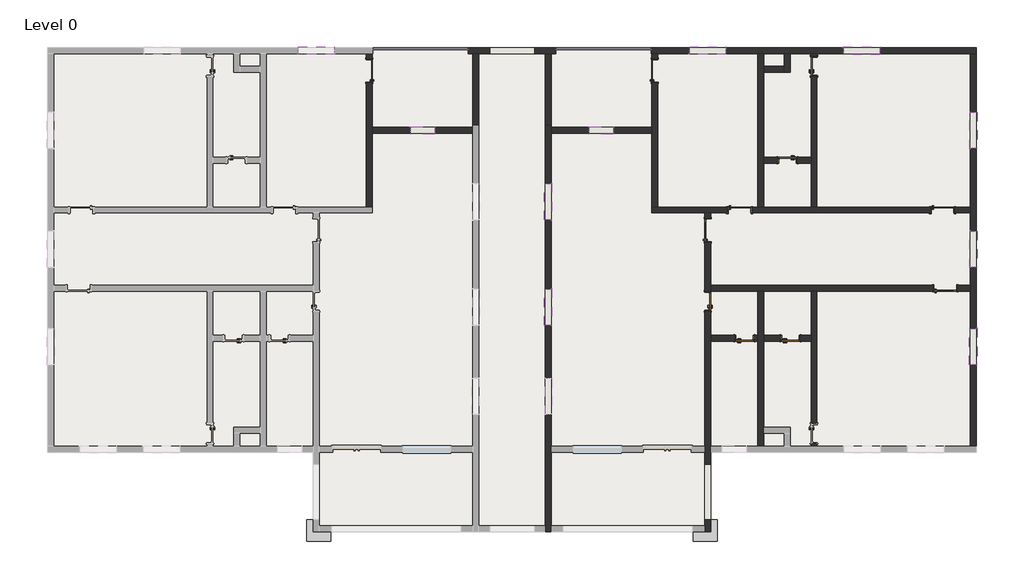
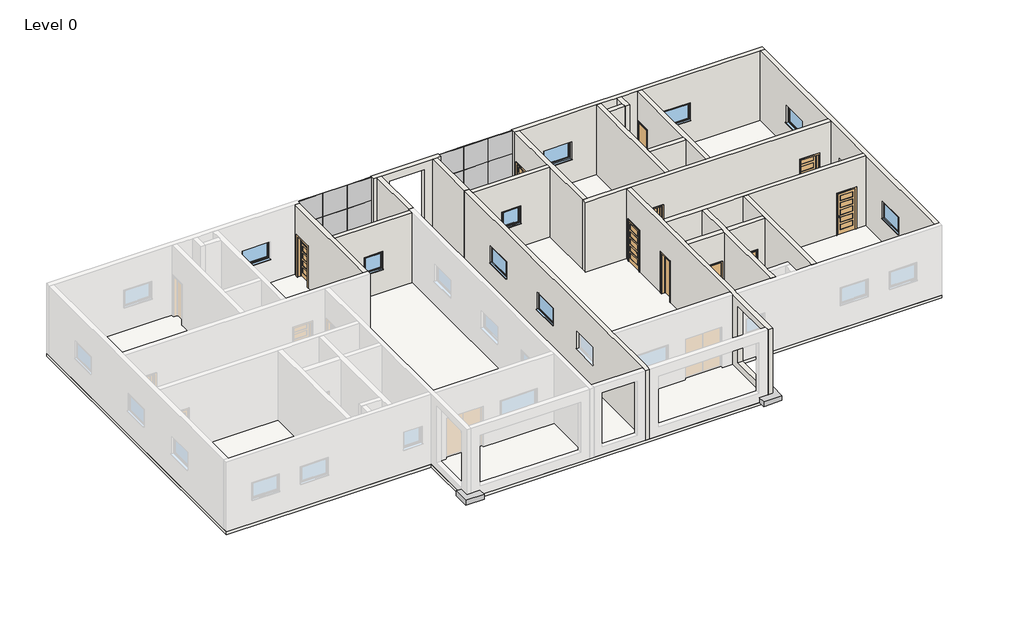
# One storey, part 2 of 2: 21 walls, 16 plates, 11 doors, 10 windows, 2 furniture elements, 1 slab.
"""IFC4 building model written with IfcOpenShell, lengths in millimetres."""

from ifc_helpers import new_model, si_unit, frame, origin, origin_with_axes, place, context, project, spatial, polyline, outline, extrude, faceted_brep, transform, mapped, element, save
from components import door_interior_single_5_panel_vert_wood_door_interior_single_0f225555, door_interior_single_5_panel_vert_wood_door_interior_single_643f6a0b, doors_intsgl_750x2110mm_542c0a28, doors_intsgl_750x2110mm_8b4efb5c, casework_1_casework_1_f5bf10af, casework_2_casework_1_9c9d669a, system_panel_glazed_6115a09f, system_panel_glazed_eff01f3a, system_panel_glazed_dd75d2a7, system_panel_glazed_dff4d0e6, system_panel_glazed_ad55aef1, system_panel_glazed_576ad081, windows_sgl_plain_1360x910mm_f5b307ae, windows_sgl_plain_1360x910mm_8a2bb76a, windows_sgl_plain_910x910mm_7835b02d, windows_sgl_plain_910x910mm_23580505

model = new_model("IFC4")

# Units and contexts
model_context = context("Model", 3, world=origin())
ifc_project = project(units=[si_unit("LENGTHUNIT", "METRE", prefix="MILLI")], contexts=[model_context])

# Site, building, storey
site = spatial("IfcSite", under=ifc_project)
building = spatial("IfcBuilding", under=site)
storey = spatial("IfcBuildingStorey", under=building, Name="Level 0", Elevation=0.0)

# Doors
placement = place(None, origin())
door_interior_single_5_panel_vert_wood_door_interior_single_shape = door_interior_single_5_panel_vert_wood_door_interior_single_0f225555(model_context)
element("IfcDoor", 1, ObjectType="Door-Interior-Single-5_Panel_Vert-Wood : Door-Interior-Single-5_Panel_Vert-Wood", at=placement, inside=storey, context=model_context, shape_type="MappedRepresentation", body=[
    mapped(door_interior_single_5_panel_vert_wood_door_interior_single_shape, transform((23913.6730929, 6189.8858821, 0.0), x_axis=(1.0, 0.0, 0.0), y_axis=(0.0, 1.0, 0.0), z_axis=(0.0, 0.0, 1.0))),
])
element("IfcDoor", 2, ObjectType="Door-Interior-Single-5_Panel_Vert-Wood : Door-Interior-Single-5_Panel_Vert-Wood", at=placement, inside=storey, context=model_context, shape_type="MappedRepresentation", body=[
    mapped(door_interior_single_5_panel_vert_wood_door_interior_single_shape, transform((31551.1730929, 6189.8858821, 0.0), x_axis=(1.0, 0.0, 0.0), y_axis=(0.0, 1.0, 0.0), z_axis=(0.0, 0.0, 1.0))),
])
element("IfcDoor", 3, ObjectType="Door-Interior-Single-5_Panel_Vert-Wood : Door-Interior-Single-5_Panel_Vert-Wood", at=placement, inside=storey, context=model_context, shape_type="MappedRepresentation", body=[
    mapped(door_interior_single_5_panel_vert_wood_door_interior_single_shape, transform((20710.4980929, 11424.2108821, 0.0), x_axis=(0.0, 1.0, 0.0), y_axis=(-1.0, 0.0, 0.0), z_axis=(0.0, 0.0, 1.0))),
])
element("IfcDoor", 4, ObjectType="Door-Interior-Single-5_Panel_Vert-Wood : Door-Interior-Single-5_Panel_Vert-Wood", at=placement, inside=storey, context=model_context, shape_type="MappedRepresentation", body=[
    mapped(door_interior_single_5_panel_vert_wood_door_interior_single_shape, transform((22710.4980929, 5424.2108821, 0.0), x_axis=(0.0, 1.0, 0.0), y_axis=(-1.0, 0.0, 0.0), z_axis=(0.0, 0.0, 1.0))),
])
door_interior_single_5_panel_vert_wood_door_interior_single_2_shape = door_interior_single_5_panel_vert_wood_door_interior_single_643f6a0b(model_context)
element("IfcDoor", 5, ObjectType="Door-Interior-Single-5_Panel_Vert-Wood : Door-Interior-Single-5_Panel_Vert-Wood", at=placement, inside=storey, context=model_context, shape_type="MappedRepresentation", body=[
    mapped(door_interior_single_5_panel_vert_wood_door_interior_single_2_shape, transform((9991.8480929, 11424.2108821, 0.0), x_axis=(0.0, 1.0, 0.0), y_axis=(-1.0, 0.0, 0.0), z_axis=(0.0, 0.0, 1.0))),
])
element("IfcDoor", 6, ObjectType="Door-Interior-Single-5_Panel_Vert-Wood : Door-Interior-Single-5_Panel_Vert-Wood", at=placement, inside=storey, context=model_context, shape_type="MappedRepresentation", body=[
    mapped(door_interior_single_5_panel_vert_wood_door_interior_single_2_shape, transform((31651.1730929, 3233.5358821, 0.0), x_axis=(1.0, 0.0, 0.0), y_axis=(0.0, 1.0, 0.0), z_axis=(0.0, 0.0, 1.0))),
])
doors_intsgl_750x2110mm_shape = doors_intsgl_750x2110mm_542c0a28(model_context)
element("IfcDoor", 7, ObjectType="Doors_IntSgl : 750x2110mm", at=placement, inside=storey, context=model_context, shape_type="MappedRepresentation", body=[
    mapped(doors_intsgl_750x2110mm_shape, transform((26713.6730929, 11599.2108821, 0.0), x_axis=(0.0, 1.0, 0.0), y_axis=(-1.0, 0.0, 0.0), z_axis=(0.0, 0.0, 1.0))),
])
doors_intsgl_750x2110mm_2_shape = doors_intsgl_750x2110mm_8b4efb5c(model_context)
element("IfcDoor", 8, ObjectType="Doors_IntSgl : 750x2110mm", at=placement, inside=storey, context=model_context, shape_type="MappedRepresentation", body=[
    mapped(doors_intsgl_750x2110mm_2_shape, transform((25713.6730929, 8061.7108821, 0.0), x_axis=(-1.0, 0.0, 0.0), y_axis=(0.0, -1.0, 0.0), z_axis=(0.0, 0.0, 1.0))),
])
element("IfcDoor", 9, ObjectType="Doors_IntSgl : 750x2110mm", at=placement, inside=storey, context=model_context, shape_type="MappedRepresentation", body=[
    mapped(doors_intsgl_750x2110mm_2_shape, transform((25826.1730929, 1361.7108821, 0.0), x_axis=(1.0, 0.0, 0.0), y_axis=(0.0, 1.0, 0.0), z_axis=(0.0, 0.0, 1.0))),
])
element("IfcDoor", 10, ObjectType="Doors_IntSgl : 750x2110mm", at=placement, inside=storey, context=model_context, shape_type="MappedRepresentation", body=[
    mapped(doors_intsgl_750x2110mm_2_shape, transform((24101.1730929, 1361.7108821, 0.0), x_axis=(1.0, 0.0, 0.0), y_axis=(0.0, 1.0, 0.0), z_axis=(0.0, 0.0, 1.0))),
])
element("IfcDoor", 11, ObjectType="Doors_IntSgl : 750x2110mm", at=placement, inside=storey, context=model_context, shape_type="MappedRepresentation", body=[
    mapped(doors_intsgl_750x2110mm_2_shape, transform((22713.6730929, 2749.2108821, 0.0), x_axis=(0.0, 1.0, 0.0), y_axis=(-1.0, 0.0, 0.0), z_axis=(0.0, 0.0, 1.0))),
])

# Furniture
casework_1_casework_1_shape = casework_1_casework_1_f5bf10af(model_context)
element("IfcFurniture", 12, ObjectType="Casework 1 : Casework 1", at=placement, inside=storey, context=model_context, shape_type="MappedRepresentation", body=[
    mapped(casework_1_casework_1_shape, transform((0.0, 0.0, 0.0), x_axis=(1.0, 0.0, 0.0), y_axis=(0.0, 1.0, 0.0), z_axis=(0.0, 0.0, 1.0))),
])
casework_2_casework_1_shape = casework_2_casework_1_9c9d669a(model_context)
element("IfcFurniture", 13, ObjectType="Casework 2 : Casework 1", at=placement, inside=storey, context=model_context, shape_type="MappedRepresentation", body=[
    mapped(casework_2_casework_1_shape, transform((0.0, 0.0, 0.0), x_axis=(1.0, 0.0, 0.0), y_axis=(0.0, 1.0, 0.0), z_axis=(0.0, 0.0, 1.0))),
])

# Plates
system_panel_glazed_shape = system_panel_glazed_6115a09f(model_context)
element("IfcPlate", 14, ObjectType="System Panel : Glazed", at=placement, inside=storey, context=model_context, shape_type="MappedRepresentation", body=[
    mapped(system_panel_glazed_shape, transform((13988.6730929, 10049.2108821, 0.0), x_axis=(0.0, 1.0, 0.0), y_axis=(-1.0, 0.0, 0.0), z_axis=(0.0, 0.0, 1.0))),
])
element("IfcPlate", 15, ObjectType="System Panel : Glazed", at=placement, inside=storey, context=model_context, shape_type="MappedRepresentation", body=[
    mapped(system_panel_glazed_shape, transform((13988.6730929, 11399.2108821, 0.0), x_axis=(0.0, 1.0, 0.0), y_axis=(-1.0, 0.0, 0.0), z_axis=(0.0, 0.0, 1.0))),
])
system_panel_glazed_2_shape = system_panel_glazed_eff01f3a(model_context)
element("IfcPlate", 16, ObjectType="System Panel : Glazed", at=placement, inside=storey, context=model_context, shape_type="MappedRepresentation", body=[
    mapped(system_panel_glazed_2_shape, transform((10717.8397596, 12186.7108821, 0.0), x_axis=(1.0, 0.0, 0.0), y_axis=(0.0, 1.0, 0.0), z_axis=(0.0, 0.0, 1.0))),
])
element("IfcPlate", 17, ObjectType="System Panel : Glazed", at=placement, inside=storey, context=model_context, shape_type="MappedRepresentation", body=[
    mapped(system_panel_glazed_2_shape, transform((11911.1730929, 12186.7108821, 0.0), x_axis=(1.0, 0.0, 0.0), y_axis=(0.0, 1.0, 0.0), z_axis=(0.0, 0.0, 1.0))),
])
element("IfcPlate", 18, ObjectType="System Panel : Glazed", at=placement, inside=storey, context=model_context, shape_type="MappedRepresentation", body=[
    mapped(system_panel_glazed_2_shape, transform((13104.5064262, 12186.7108821, 0.0), x_axis=(1.0, 0.0, 0.0), y_axis=(0.0, 1.0, 0.0), z_axis=(0.0, 0.0, 1.0))),
])
system_panel_glazed_3_shape = system_panel_glazed_dd75d2a7(model_context)
element("IfcPlate", 19, ObjectType="System Panel : Glazed", at=placement, inside=storey, context=model_context, shape_type="MappedRepresentation", body=[
    mapped(system_panel_glazed_3_shape, transform((10717.8397596, 12186.7108821, 2400.0), x_axis=(1.0, 0.0, 0.0), y_axis=(0.0, 1.0, 0.0), z_axis=(0.0, 0.0, 1.0))),
])
element("IfcPlate", 20, ObjectType="System Panel : Glazed", at=placement, inside=storey, context=model_context, shape_type="MappedRepresentation", body=[
    mapped(system_panel_glazed_3_shape, transform((11911.1730929, 12186.7108821, 2400.0), x_axis=(1.0, 0.0, 0.0), y_axis=(0.0, 1.0, 0.0), z_axis=(0.0, 0.0, 1.0))),
])
element("IfcPlate", 21, ObjectType="System Panel : Glazed", at=placement, inside=storey, context=model_context, shape_type="MappedRepresentation", body=[
    mapped(system_panel_glazed_3_shape, transform((13104.5064262, 12186.7108821, 2400.0), x_axis=(1.0, 0.0, 0.0), y_axis=(0.0, 1.0, 0.0), z_axis=(0.0, 0.0, 1.0))),
])
system_panel_glazed_4_shape = system_panel_glazed_dff4d0e6(model_context)
element("IfcPlate", 22, ObjectType="System Panel : Glazed", at=placement, inside=storey, context=model_context, shape_type="MappedRepresentation", body=[
    mapped(system_panel_glazed_4_shape, transform((16713.6730929, 10049.2108821, 0.0), x_axis=(0.0, 1.0, 0.0), y_axis=(-1.0, 0.0, 0.0), z_axis=(0.0, 0.0, 1.0))),
])
element("IfcPlate", 23, ObjectType="System Panel : Glazed", at=placement, inside=storey, context=model_context, shape_type="MappedRepresentation", body=[
    mapped(system_panel_glazed_4_shape, transform((16713.6730929, 11399.2108821, 0.0), x_axis=(0.0, 1.0, 0.0), y_axis=(-1.0, 0.0, 0.0), z_axis=(0.0, 0.0, 1.0))),
])
system_panel_glazed_5_shape = system_panel_glazed_ad55aef1(model_context)
element("IfcPlate", 24, ObjectType="System Panel : Glazed", at=placement, inside=storey, context=model_context, shape_type="MappedRepresentation", body=[
    mapped(system_panel_glazed_5_shape, transform((19984.5064262, 12186.7108821, 0.0), x_axis=(-1.0, 0.0, 0.0), y_axis=(0.0, -1.0, 0.0), z_axis=(0.0, 0.0, 1.0))),
])
element("IfcPlate", 25, ObjectType="System Panel : Glazed", at=placement, inside=storey, context=model_context, shape_type="MappedRepresentation", body=[
    mapped(system_panel_glazed_5_shape, transform((18791.1730929, 12186.7108821, 0.0), x_axis=(-1.0, 0.0, 0.0), y_axis=(0.0, -1.0, 0.0), z_axis=(0.0, 0.0, 1.0))),
])
element("IfcPlate", 26, ObjectType="System Panel : Glazed", at=placement, inside=storey, context=model_context, shape_type="MappedRepresentation", body=[
    mapped(system_panel_glazed_5_shape, transform((17597.8397596, 12186.7108821, 0.0), x_axis=(-1.0, 0.0, 0.0), y_axis=(0.0, -1.0, 0.0), z_axis=(0.0, 0.0, 1.0))),
])
system_panel_glazed_6_shape = system_panel_glazed_576ad081(model_context)
element("IfcPlate", 27, ObjectType="System Panel : Glazed", at=placement, inside=storey, context=model_context, shape_type="MappedRepresentation", body=[
    mapped(system_panel_glazed_6_shape, transform((19984.5064262, 12186.7108821, 2400.0), x_axis=(-1.0, 0.0, 0.0), y_axis=(0.0, -1.0, 0.0), z_axis=(0.0, 0.0, 1.0))),
])
element("IfcPlate", 28, ObjectType="System Panel : Glazed", at=placement, inside=storey, context=model_context, shape_type="MappedRepresentation", body=[
    mapped(system_panel_glazed_6_shape, transform((18791.1730929, 12186.7108821, 2400.0), x_axis=(-1.0, 0.0, 0.0), y_axis=(0.0, -1.0, 0.0), z_axis=(0.0, 0.0, 1.0))),
])
element("IfcPlate", 29, ObjectType="System Panel : Glazed", at=placement, inside=storey, context=model_context, shape_type="MappedRepresentation", body=[
    mapped(system_panel_glazed_6_shape, transform((17597.8397596, 12186.7108821, 2400.0), x_axis=(-1.0, 0.0, 0.0), y_axis=(0.0, -1.0, 0.0), z_axis=(0.0, 0.0, 1.0))),
])

# Slab
element("IfcSlab", 30, ObjectType="Floor-Grnd-Susp_65Scr-80Ins-100Blk-75PC", at=placement, inside=storey, context=model_context, shape_type="SweptSolid", body=[
    extrude(outline(polyline([(-2123.8269071, -2925.7891179), (-2123.8269071, 12299.2108821), (15317.0017019, 12299.2108821), (15484.4665966, 12299.2108821), (32826.1730929, 12299.2108821), (32826.1730929, -2925.7891179), (22826.1730929, -2925.7891179), (22826.1730929, -5925.7891179), (7876.1730929, -5925.7891179), (7876.1730929, -2925.7891179), (-2123.8269071, -2925.7891179)])), frame((0.0, 0.0, -150.0), z_axis=(0.0, 0.0, 1.0), x_axis=(1.0, 0.0, 0.0)), (0.0, 0.0, 1.0), 150.0),
])

# Walls
element("IfcWall", 31, ObjectType="GENERIC 225", at=placement, inside=storey, context=model_context, shape_type="SweptSolid", body=[
    extrude(outline(polyline([(13876.1730929, 9374.2108821), (13876.1730929, 12074.2108821), (14101.1730929, 12074.2108821), (14101.1730929, 9374.2108821), (13876.1730929, 9374.2108821)])), origin_with_axes(), (0.0, 0.0, 1.0), 3600.0),
])
element("IfcWall", 32, ObjectType="GENERIC 225", at=placement, inside=storey, context=model_context, shape_type="Brep", body=[
    faceted_brep([(10101.1730929, 12074.2108821, 3600.0), (10101.1730929, 9299.2108821, 3600.0), (10101.1730929, 9074.2108821, 3600.0), (10101.1730929, 6299.2108821, 3600.0), (10101.1730929, 6299.2108821, 0.0), (10101.1730929, 9074.2108821, 0.0), (10101.1730929, 9299.2108821, 0.0), (10101.1730929, 10974.2108821, 0.0), (10101.1730929, 10974.2108821, 2125.4), (10101.1730929, 11874.2108821, 2125.4), (10101.1730929, 11874.2108821, 0.0), (10101.1730929, 12074.2108821, 0.0), (9876.1730929, 6299.2108821, 3600.0), (9876.1730929, 12074.2108821, 3600.0), (9876.1730929, 12074.2108821, 0.0), (9876.1730929, 11874.2108821, 0.0), (9876.1730929, 11874.2108821, 2125.4), (9876.1730929, 10974.2108821, 2125.4), (9876.1730929, 10974.2108821, 0.0), (9876.1730929, 6299.2108821, 0.0)], [[[0, 1, 2, 3, 4, 5, 6, 7, 8, 9, 10, 11]], [[12, 13, 14, 15, 16, 17, 18, 19]], [[4, 19, 18, 7, 6, 5]], [[14, 11, 10, 15]], [[3, 2, 1, 0, 13, 12]], [[4, 3, 12, 19]], [[0, 11, 14, 13]], [[9, 16, 15, 10]], [[16, 9, 8, 17]], [[17, 8, 7, 18]]]),
])
element("IfcWall", 33, ObjectType="GENERIC 225", at=placement, inside=storey, context=model_context, shape_type="SweptSolid", body=[
    extrude(outline(polyline([(0.0, 13876.1730929), (3600.0, 13876.1730929), (3600.0, 10101.1730929), (0.0, 10101.1730929), (0.0, 13876.1730929)]), holes=[polyline([(2110.0, 12443.6730929), (1200.0, 12443.6730929), (1200.0, 11533.6730929), (2110.0, 11533.6730929), (2110.0, 12443.6730929)])]), frame((0.0, 9074.2108821, 0.0), z_axis=(0.0, 1.0, 0.0), x_axis=(0.0, 0.0, 1.0)), (0.0, 0.0, 1.0), 225.0),
])
element("IfcWall", 34, ObjectType="GENERIC 225", at=placement, inside=storey, context=model_context, shape_type="Brep", body=[
    faceted_brep([(32826.1730929, 12299.2108821, 0.0), (20581.1730929, 12299.2108821, 0.0), (20581.1730929, 12299.2108821, 3600.0), (32826.1730929, 12299.2108821, 3600.0), (27826.1730929, 12299.2108821, 2110.0), (27826.1730929, 12299.2108821, 1200.0), (29186.1730929, 12299.2108821, 1200.0), (29186.1730929, 12299.2108821, 2110.0), (23393.6730929, 12299.2108821, 2110.0), (22033.6730929, 12299.2108821, 2110.0), (22033.6730929, 12299.2108821, 1200.0), (23393.6730929, 12299.2108821, 1200.0), (32826.1730929, 12074.2108821, 0.0), (32826.1730929, 12074.2108821, 3600.0), (32601.1730929, 12074.2108821, 3600.0), (26826.1730929, 12074.2108821, 3600.0), (26601.1730929, 12074.2108821, 3600.0), (25826.1730929, 12074.2108821, 3600.0), (25601.1730929, 12074.2108821, 3600.0), (24826.1730929, 12074.2108821, 3600.0), (24601.1730929, 12074.2108821, 3600.0), (20826.1730929, 12074.2108821, 3600.0), (20601.1730929, 12074.2108821, 3600.0), (20581.1730929, 12074.2108821, 3600.0), (20581.1730929, 12074.2108821, 0.0), (20601.1730929, 12074.2108821, 0.0), (20826.1730929, 12074.2108821, 0.0), (24601.1730929, 12074.2108821, 0.0), (24826.1730929, 12074.2108821, 0.0), (25601.1730929, 12074.2108821, 0.0), (25826.1730929, 12074.2108821, 0.0), (26601.1730929, 12074.2108821, 0.0), (26826.1730929, 12074.2108821, 0.0), (32601.1730929, 12074.2108821, 0.0), (27826.1730929, 12074.2108821, 2110.0), (29186.1730929, 12074.2108821, 2110.0), (29186.1730929, 12074.2108821, 1200.0), (27826.1730929, 12074.2108821, 1200.0), (23393.6730929, 12074.2108821, 2110.0), (23393.6730929, 12074.2108821, 1200.0), (22033.6730929, 12074.2108821, 1200.0), (22033.6730929, 12074.2108821, 2110.0)], [[[0, 1, 2, 3], [4, 5, 6, 7], [8, 9, 10, 11]], [[12, 13, 14, 15, 16, 17, 18, 19, 20, 21, 22, 23, 24, 25, 26, 27, 28, 29, 30, 31, 32, 33], [34, 35, 36, 37], [38, 39, 40, 41]], [[1, 0, 12, 33, 32, 31, 30, 29, 28, 27, 26, 25, 24]], [[2, 1, 24, 23]], [[3, 2, 23, 22, 21, 20, 19, 18, 17, 16, 15, 14, 13]], [[0, 3, 13, 12]], [[5, 4, 34, 37]], [[6, 5, 37, 36]], [[7, 6, 36, 35]], [[4, 7, 35, 34]], [[39, 38, 8, 11]], [[40, 39, 11, 10]], [[41, 40, 10, 9]], [[38, 41, 9, 8]]]),
])
element("IfcWall", 35, ObjectType="GENERIC 225", at=placement, inside=storey, context=model_context, shape_type="SweptSolid", body=[
    extrude(outline(polyline([(16601.1730929, 9374.2108821), (16601.1730929, 12074.2108821), (16826.1730929, 12074.2108821), (16826.1730929, 9374.2108821), (16601.1730929, 9374.2108821)])), origin_with_axes(), (0.0, 0.0, 1.0), 3600.0),
])
element("IfcWall", 36, ObjectType="GENERIC 225", at=placement, inside=storey, context=model_context, shape_type="Brep", body=[
    faceted_brep([(22826.1730929, 6074.2108821, 3600.0), (22826.1730929, 3349.2108821, 3600.0), (22826.1730929, 3124.2108821, 3600.0), (22826.1730929, 1474.2108821, 3600.0), (22826.1730929, 1249.2108821, 3600.0), (22826.1730929, -2700.7891179, 3600.0), (22826.1730929, -2925.7891179, 3600.0), (22826.1730929, -5925.7891179, 3600.0), (22826.1730929, -5925.7891179, 0.0), (22826.1730929, -2925.7891179, 0.0), (22826.1730929, -2700.7891179, 0.0), (22826.1730929, 1249.2108821, 0.0), (22826.1730929, 1474.2108821, 0.0), (22826.1730929, 2374.2108821, 0.0), (22826.1730929, 2374.2108821, 2110.0), (22826.1730929, 3124.2108821, 2110.0), (22826.1730929, 3124.2108821, 0.0), (22826.1730929, 3349.2108821, 0.0), (22826.1730929, 4974.2108821, 0.0), (22826.1730929, 4974.2108821, 2125.4), (22826.1730929, 5874.2108821, 2125.4), (22826.1730929, 5874.2108821, 0.0), (22826.1730929, 6074.2108821, 0.0), (22826.1730929, -5475.2269163, 3254.1937526), (22826.1730929, -3375.2269163, 3254.1937526), (22826.1730929, -3375.2269163, 354.1937526), (22826.1730929, -5475.2269163, 354.1937526), (22601.1730929, -5925.7891179, 3600.0), (22601.1730929, -5700.7891179, 3600.0), (22601.1730929, -2925.7891179, 3600.0), (22601.1730929, -2700.7891179, 3600.0), (22601.1730929, 6074.2108821, 3600.0), (22601.1730929, 6074.2108821, 0.0), (22601.1730929, 5874.2108821, 0.0), (22601.1730929, 5874.2108821, 2125.4), (22601.1730929, 4974.2108821, 2125.4), (22601.1730929, 4974.2108821, 0.0), (22601.1730929, 3124.2108821, 0.0), (22601.1730929, 3124.2108821, 2110.0), (22601.1730929, 2374.2108821, 2110.0), (22601.1730929, 2374.2108821, 0.0), (22601.1730929, -2700.7891179, 0.0), (22601.1730929, -2925.7891179, 0.0), (22601.1730929, -5700.7891179, 0.0), (22601.1730929, -5925.7891179, 0.0), (22601.1730929, -3375.2269163, 3254.1937526), (22601.1730929, -5475.2269163, 3254.1937526), (22601.1730929, -5475.2269163, 354.1937526), (22601.1730929, -3375.2269163, 354.1937526)], [[[0, 1, 2, 3, 4, 5, 6, 7, 8, 9, 10, 11, 12, 13, 14, 15, 16, 17, 18, 19, 20, 21, 22], [23, 24, 25, 26]], [[27, 28, 29, 30, 31, 32, 33, 34, 35, 36, 37, 38, 39, 40, 41, 42, 43, 44], [45, 46, 47, 48]], [[0, 22, 32, 31]], [[20, 34, 33, 21]], [[34, 20, 19, 35]], [[35, 19, 18, 36]], [[15, 38, 37, 16]], [[38, 15, 14, 39]], [[39, 14, 13, 40]], [[8, 7, 27, 44]], [[22, 21, 33, 32]], [[8, 44, 43, 42, 41, 40, 13, 12, 11, 10, 9]], [[36, 18, 17, 16, 37]], [[7, 6, 5, 4, 3, 2, 1, 0, 31, 30, 29, 28, 27]], [[24, 23, 46, 45]], [[25, 24, 45, 48]], [[26, 25, 48, 47]], [[23, 26, 47, 46]]]),
])
element("IfcWall", 37, ObjectType="GENERIC 225", at=placement, inside=storey, context=model_context, shape_type="Brep", body=[
    faceted_brep([(32826.1730929, -2700.7891179, 0.0), (32826.1730929, 12074.2108821, 0.0), (32826.1730929, 12074.2108821, 3600.0), (32826.1730929, -2700.7891179, 3600.0), (32826.1730929, 8506.7108821, 2110.0), (32826.1730929, 9866.7108821, 2110.0), (32826.1730929, 9866.7108821, 1200.0), (32826.1730929, 8506.7108821, 1200.0), (32826.1730929, 4031.7108821, 2110.0), (32826.1730929, 5391.7108821, 2110.0), (32826.1730929, 5391.7108821, 1200.0), (32826.1730929, 4031.7108821, 1200.0), (32826.1730929, 1724.2108821, 2110.0), (32826.1730929, 1724.2108821, 1200.0), (32826.1730929, 364.2108821, 1200.0), (32826.1730929, 364.2108821, 2110.0), (32601.1730929, -2700.7891179, 0.0), (32601.1730929, -2700.7891179, 3600.0), (32601.1730929, 3124.2108821, 3600.0), (32601.1730929, 3349.2108821, 3600.0), (32601.1730929, 6074.2108821, 3600.0), (32601.1730929, 6299.2108821, 3600.0), (32601.1730929, 12074.2108821, 3600.0), (32601.1730929, 12074.2108821, 0.0), (32601.1730929, 6299.2108821, 0.0), (32601.1730929, 6074.2108821, 0.0), (32601.1730929, 3349.2108821, 0.0), (32601.1730929, 3124.2108821, 0.0), (32601.1730929, 8506.7108821, 2110.0), (32601.1730929, 8506.7108821, 1200.0), (32601.1730929, 9866.7108821, 1200.0), (32601.1730929, 9866.7108821, 2110.0), (32601.1730929, 4031.7108821, 2110.0), (32601.1730929, 4031.7108821, 1200.0), (32601.1730929, 5391.7108821, 1200.0), (32601.1730929, 5391.7108821, 2110.0), (32601.1730929, 1724.2108821, 2110.0), (32601.1730929, 364.2108821, 2110.0), (32601.1730929, 364.2108821, 1200.0), (32601.1730929, 1724.2108821, 1200.0)], [[[0, 1, 2, 3], [4, 5, 6, 7], [8, 9, 10, 11], [12, 13, 14, 15]], [[16, 17, 18, 19, 20, 21, 22, 23, 24, 25, 26, 27], [28, 29, 30, 31], [32, 33, 34, 35], [36, 37, 38, 39]], [[1, 0, 16, 27, 26, 25, 24, 23]], [[3, 2, 22, 21, 20, 19, 18, 17]], [[2, 1, 23, 22]], [[0, 3, 17, 16]], [[29, 28, 4, 7]], [[30, 29, 7, 6]], [[31, 30, 6, 5]], [[28, 31, 5, 4]], [[33, 32, 8, 11]], [[34, 33, 11, 10]], [[35, 34, 10, 9]], [[32, 35, 9, 8]], [[13, 12, 36, 39]], [[14, 13, 39, 38]], [[15, 14, 38, 37]], [[12, 15, 37, 36]]]),
])
element("IfcWall", 38, ObjectType="GENERIC 225", at=placement, inside=storey, context=model_context, shape_type="Brep", body=[
    faceted_brep([(22826.1730929, 3349.2108821, 3600.0), (32601.1730929, 3349.2108821, 3600.0), (32601.1730929, 3349.2108821, 0.0), (32101.1730929, 3349.2108821, 0.0), (32101.1730929, 3349.2108821, 2125.4), (31201.1730929, 3349.2108821, 2125.4), (31201.1730929, 3349.2108821, 0.0), (22826.1730929, 3349.2108821, 0.0), (32601.1730929, 3124.2108821, 3600.0), (26826.1730929, 3124.2108821, 3600.0), (26601.1730929, 3124.2108821, 3600.0), (24826.1730929, 3124.2108821, 3600.0), (24601.1730929, 3124.2108821, 3600.0), (22826.1730929, 3124.2108821, 3600.0), (22826.1730929, 3124.2108821, 2110.0), (22826.1730929, 3124.2108821, 0.0), (24601.1730929, 3124.2108821, 0.0), (24826.1730929, 3124.2108821, 0.0), (26601.1730929, 3124.2108821, 0.0), (26826.1730929, 3124.2108821, 0.0), (31201.1730929, 3124.2108821, 0.0), (31201.1730929, 3124.2108821, 2125.4), (32101.1730929, 3124.2108821, 2125.4), (32101.1730929, 3124.2108821, 0.0), (32601.1730929, 3124.2108821, 0.0)], [[[0, 1, 2, 3, 4, 5, 6, 7]], [[8, 9, 10, 11, 12, 13, 14, 15, 16, 17, 18, 19, 20, 21, 22, 23, 24]], [[2, 24, 23, 3]], [[15, 7, 6, 20, 19, 18, 17, 16]], [[1, 0, 13, 12, 11, 10, 9, 8]], [[2, 1, 8, 24]], [[0, 7, 15, 14, 13]], [[22, 4, 3, 23]], [[4, 22, 21, 5]], [[5, 21, 20, 6]]]),
])
element("IfcWall", 39, ObjectType="GENERIC 225", at=placement, inside=storey, context=model_context, shape_type="Brep", body=[
    faceted_brep([(26601.1730929, -2700.7891179, 3600.0), (26601.1730929, 1249.2108821, 3600.0), (26601.1730929, 1474.2108821, 3600.0), (26601.1730929, 3124.2108821, 3600.0), (26601.1730929, 3124.2108821, 0.0), (26601.1730929, 1474.2108821, 0.0), (26601.1730929, 1249.2108821, 0.0), (26601.1730929, -1850.7891179, 0.0), (26601.1730929, -1850.7891179, 2110.0), (26601.1730929, -2600.7891179, 2110.0), (26601.1730929, -2600.7891179, 0.0), (26601.1730929, -2700.7891179, 0.0), (26826.1730929, 3124.2108821, 3600.0), (26826.1730929, -2700.7891179, 3600.0), (26826.1730929, -2700.7891179, 0.0), (26826.1730929, -2600.7891179, 0.0), (26826.1730929, -2600.7891179, 2110.0), (26826.1730929, -1850.7891179, 2110.0), (26826.1730929, -1850.7891179, 0.0), (26826.1730929, 3124.2108821, 0.0)], [[[0, 1, 2, 3, 4, 5, 6, 7, 8, 9, 10, 11]], [[12, 13, 14, 15, 16, 17, 18, 19]], [[4, 19, 18, 7, 6, 5]], [[14, 11, 10, 15]], [[3, 2, 1, 0, 13, 12]], [[4, 3, 12, 19]], [[0, 11, 14, 13]], [[9, 16, 15, 10]], [[16, 9, 8, 17]], [[17, 8, 7, 18]]]),
])
element("IfcWall", 40, ObjectType="GENERIC 225", at=placement, inside=storey, context=model_context, shape_type="Brep", body=[
    faceted_brep([(20601.1730929, 6299.2108821, 3600.0), (20826.1730929, 6299.2108821, 3600.0), (24601.1730929, 6299.2108821, 3600.0), (24826.1730929, 6299.2108821, 3600.0), (26601.1730929, 6299.2108821, 3600.0), (26826.1730929, 6299.2108821, 3600.0), (32601.1730929, 6299.2108821, 3600.0), (32601.1730929, 6299.2108821, 0.0), (32001.1730929, 6299.2108821, 0.0), (32001.1730929, 6299.2108821, 2125.4), (31101.1730929, 6299.2108821, 2125.4), (31101.1730929, 6299.2108821, 0.0), (26826.1730929, 6299.2108821, 0.0), (26601.1730929, 6299.2108821, 0.0), (24826.1730929, 6299.2108821, 0.0), (24601.1730929, 6299.2108821, 0.0), (24363.6730929, 6299.2108821, 0.0), (24363.6730929, 6299.2108821, 2125.4), (23463.6730929, 6299.2108821, 2125.4), (23463.6730929, 6299.2108821, 0.0), (20826.1730929, 6299.2108821, 0.0), (20601.1730929, 6299.2108821, 0.0), (32601.1730929, 6074.2108821, 3600.0), (22826.1730929, 6074.2108821, 3600.0), (22601.1730929, 6074.2108821, 3600.0), (20601.1730929, 6074.2108821, 3600.0), (20601.1730929, 6074.2108821, 0.0), (22601.1730929, 6074.2108821, 0.0), (22826.1730929, 6074.2108821, 0.0), (23463.6730929, 6074.2108821, 0.0), (23463.6730929, 6074.2108821, 2125.4), (24363.6730929, 6074.2108821, 2125.4), (24363.6730929, 6074.2108821, 0.0), (31101.1730929, 6074.2108821, 0.0), (31101.1730929, 6074.2108821, 2125.4), (32001.1730929, 6074.2108821, 2125.4), (32001.1730929, 6074.2108821, 0.0), (32601.1730929, 6074.2108821, 0.0)], [[[0, 1, 2, 3, 4, 5, 6, 7, 8, 9, 10, 11, 12, 13, 14, 15, 16, 17, 18, 19, 20, 21]], [[22, 23, 24, 25, 26, 27, 28, 29, 30, 31, 32, 33, 34, 35, 36, 37]], [[7, 37, 36, 8]], [[26, 21, 20, 19, 29, 28, 27]], [[32, 16, 15, 14, 13, 12, 11, 33]], [[6, 5, 4, 3, 2, 1, 0, 25, 24, 23, 22]], [[7, 6, 22, 37]], [[0, 21, 26, 25]], [[17, 16, 32, 31]], [[18, 17, 31, 30]], [[19, 18, 30, 29]], [[35, 9, 8, 36]], [[9, 35, 34, 10]], [[10, 34, 33, 11]]]),
])
element("IfcWall", 41, ObjectType="GENERIC 225", at=placement, inside=storey, context=model_context, shape_type="Brep", body=[
    faceted_brep([(26826.1730929, 12074.2108821, 3600.0), (26826.1730929, 6299.2108821, 3600.0), (26826.1730929, 6299.2108821, 0.0), (26826.1730929, 11224.2108821, 0.0), (26826.1730929, 11224.2108821, 2110.0), (26826.1730929, 11974.2108821, 2110.0), (26826.1730929, 11974.2108821, 0.0), (26826.1730929, 12074.2108821, 0.0), (26601.1730929, 6299.2108821, 3600.0), (26601.1730929, 7949.2108821, 3600.0), (26601.1730929, 8174.2108821, 3600.0), (26601.1730929, 12074.2108821, 3600.0), (26601.1730929, 12074.2108821, 0.0), (26601.1730929, 11974.2108821, 0.0), (26601.1730929, 11974.2108821, 2110.0), (26601.1730929, 11224.2108821, 2110.0), (26601.1730929, 11224.2108821, 0.0), (26601.1730929, 8174.2108821, 0.0), (26601.1730929, 7949.2108821, 0.0), (26601.1730929, 6299.2108821, 0.0)], [[[0, 1, 2, 3, 4, 5, 6, 7]], [[8, 9, 10, 11, 12, 13, 14, 15, 16, 17, 18, 19]], [[2, 19, 18, 17, 16, 3]], [[12, 7, 6, 13]], [[1, 0, 11, 10, 9, 8]], [[2, 1, 8, 19]], [[0, 7, 12, 11]], [[5, 14, 13, 6]], [[14, 5, 4, 15]], [[15, 4, 3, 16]]]),
])
element("IfcWall", 42, ObjectType="GENERIC 225", at=placement, inside=storey, context=model_context, shape_type="Brep", body=[
    faceted_brep([(20826.1730929, 12074.2108821, 3600.0), (20826.1730929, 6299.2108821, 3600.0), (20826.1730929, 6299.2108821, 0.0), (20826.1730929, 10974.2108821, 0.0), (20826.1730929, 10974.2108821, 2125.4), (20826.1730929, 11874.2108821, 2125.4), (20826.1730929, 11874.2108821, 0.0), (20826.1730929, 12074.2108821, 0.0), (20601.1730929, 6299.2108821, 3600.0), (20601.1730929, 9074.2108821, 3600.0), (20601.1730929, 9299.2108821, 3600.0), (20601.1730929, 12074.2108821, 3600.0), (20601.1730929, 12074.2108821, 0.0), (20601.1730929, 11874.2108821, 0.0), (20601.1730929, 11874.2108821, 2125.4), (20601.1730929, 10974.2108821, 2125.4), (20601.1730929, 10974.2108821, 0.0), (20601.1730929, 9299.2108821, 0.0), (20601.1730929, 9074.2108821, 0.0), (20601.1730929, 6299.2108821, 0.0)], [[[0, 1, 2, 3, 4, 5, 6, 7]], [[8, 9, 10, 11, 12, 13, 14, 15, 16, 17, 18, 19]], [[2, 19, 18, 17, 16, 3]], [[12, 7, 6, 13]], [[1, 0, 11, 10, 9, 8]], [[2, 1, 8, 19]], [[0, 7, 12, 11]], [[5, 14, 13, 6]], [[14, 5, 4, 15]], [[15, 4, 3, 16]]]),
])
element("IfcWall", 43, ObjectType="GENERIC 225", at=placement, inside=storey, context=model_context, shape_type="SweptSolid", body=[
    extrude(outline(polyline([(0.0, 16826.1730929), (0.0, 20601.1730929), (3600.0, 20601.1730929), (3600.0, 16826.1730929), (0.0, 16826.1730929)]), holes=[polyline([(2110.0, 18258.6730929), (2110.0, 19168.6730929), (1200.0, 19168.6730929), (1200.0, 18258.6730929), (2110.0, 18258.6730929)])]), frame((0.0, 9074.2108821, 0.0), z_axis=(0.0, 1.0, 0.0), x_axis=(0.0, 0.0, 1.0)), (0.0, 0.0, 1.0), 225.0),
])
element("IfcWall", 44, ObjectType="GENERIC 225", at=placement, inside=storey, context=model_context, shape_type="Brep", body=[
    faceted_brep([(24601.1730929, 3124.2108821, 0.0), (24601.1730929, 1474.2108821, 0.0), (24601.1730929, 1249.2108821, 0.0), (24601.1730929, -2700.7891179, 0.0), (24601.1730929, -2700.7891179, 3600.0), (24601.1730929, 1249.2108821, 3600.0), (24601.1730929, 1474.2108821, 3600.0), (24601.1730929, 3124.2108821, 3600.0), (24826.1730929, 3124.2108821, 0.0), (24826.1730929, 3124.2108821, 3600.0), (24826.1730929, 1474.2108821, 3600.0), (24826.1730929, 1249.2108821, 3600.0), (24826.1730929, -1988.2891179, 3600.0), (24826.1730929, -2213.2891179, 3600.0), (24826.1730929, -2700.7891179, 3600.0), (24826.1730929, -2700.7891179, 0.0), (24826.1730929, -2213.2891179, 0.0), (24826.1730929, -1988.2891179, 0.0), (24826.1730929, 1249.2108821, 0.0), (24826.1730929, 1474.2108821, 0.0)], [[[0, 1, 2, 3, 4, 5, 6, 7]], [[8, 9, 10, 11, 12, 13, 14, 15, 16, 17, 18, 19]], [[3, 2, 1, 0, 8, 19, 18, 17, 16, 15]], [[7, 6, 5, 4, 14, 13, 12, 11, 10, 9]], [[4, 3, 15, 14]], [[0, 7, 9, 8]]]),
])
element("IfcWall", 45, ObjectType="GENERIC 225", at=placement, inside=storey, context=model_context, shape_type="Brep", body=[
    faceted_brep([(24601.1730929, 12074.2108821, 0.0), (24601.1730929, 6299.2108821, 0.0), (24601.1730929, 6299.2108821, 3600.0), (24601.1730929, 12074.2108821, 3600.0), (24826.1730929, 12074.2108821, 0.0), (24826.1730929, 12074.2108821, 3600.0), (24826.1730929, 11599.2108821, 3600.0), (24826.1730929, 11374.2108821, 3600.0), (24826.1730929, 8174.2108821, 3600.0), (24826.1730929, 7949.2108821, 3600.0), (24826.1730929, 6299.2108821, 3600.0), (24826.1730929, 6299.2108821, 0.0), (24826.1730929, 7949.2108821, 0.0), (24826.1730929, 8174.2108821, 0.0), (24826.1730929, 11374.2108821, 0.0), (24826.1730929, 11599.2108821, 0.0)], [[[0, 1, 2, 3]], [[4, 5, 6, 7, 8, 9, 10, 11, 12, 13, 14, 15]], [[1, 0, 4, 15, 14, 13, 12, 11]], [[3, 2, 10, 9, 8, 7, 6, 5]], [[0, 3, 5, 4]], [[2, 1, 11, 10]]]),
])
element("IfcWall", 46, ObjectType="GENERIC 225", at=placement, inside=storey, context=model_context, shape_type="SweptSolid", body=[
    extrude(outline(polyline([(3600.0, 26601.1730929), (3600.0, 24826.1730929), (0.0, 24826.1730929), (0.0, 25338.6730929), (2110.0, 25338.6730929), (2110.0, 26088.6730929), (0.0, 26088.6730929), (0.0, 26601.1730929), (3600.0, 26601.1730929)])), frame((0.0, 7949.2108821, 0.0), z_axis=(0.0, 1.0, 0.0), x_axis=(0.0, 0.0, 1.0)), (0.0, 0.0, 1.0), 225.0),
])
element("IfcWall", 47, ObjectType="GENERIC 225", at=placement, inside=storey, context=model_context, shape_type="SweptSolid", body=[
    extrude(outline(polyline([(3600.0, 22826.1730929), (0.0, 22826.1730929), (0.0, 23726.1730929), (2110.0, 23726.1730929), (2110.0, 24476.1730929), (0.0, 24476.1730929), (0.0, 24601.1730929), (3600.0, 24601.1730929), (3600.0, 22826.1730929)])), frame((0.0, 1249.2108821, 0.0), z_axis=(0.0, 1.0, 0.0), x_axis=(0.0, 0.0, 1.0)), (0.0, 0.0, 1.0), 225.0),
    extrude(outline(polyline([(0.0, 26601.1730929), (3600.0, 26601.1730929), (3600.0, 24826.1730929), (0.0, 24826.1730929), (0.0, 25451.1730929), (2110.0, 25451.1730929), (2110.0, 26201.1730929), (0.0, 26201.1730929), (0.0, 26601.1730929)])), frame((0.0, 1249.2108821, 0.0), z_axis=(0.0, 1.0, 0.0), x_axis=(0.0, 0.0, 1.0)), (0.0, 0.0, 1.0), 225.0),
])
element("IfcWall", 48, ObjectType="GENERIC 225", at=placement, inside=storey, context=model_context, shape_type="Brep", body=[
    faceted_brep([(25601.1730929, 12074.2108821, 0.0), (25601.1730929, 11599.2108821, 0.0), (25601.1730929, 11374.2108821, 0.0), (25601.1730929, 11374.2108821, 3600.0), (25601.1730929, 11599.2108821, 3600.0), (25601.1730929, 12074.2108821, 3600.0), (25826.1730929, 12074.2108821, 0.0), (25826.1730929, 12074.2108821, 3600.0), (25826.1730929, 11374.2108821, 3600.0), (25826.1730929, 11374.2108821, 0.0)], [[[0, 1, 2, 3, 4, 5]], [[6, 7, 8, 9]], [[2, 1, 0, 6, 9]], [[5, 4, 3, 8, 7]], [[0, 5, 7, 6]], [[3, 2, 9, 8]]]),
])
element("IfcWall", 49, ObjectType="GENERIC 225", at=placement, inside=storey, context=model_context, shape_type="SweptSolid", body=[
    extrude(outline(polyline([(24826.1730929, 11599.2108821), (25601.1730929, 11599.2108821), (25601.1730929, 11374.2108821), (24826.1730929, 11374.2108821), (24826.1730929, 11599.2108821)])), origin_with_axes(), (0.0, 0.0, 1.0), 3600.0),
])
element("IfcWall", 50, ObjectType="GENERIC 225", at=placement, inside=storey, context=model_context, shape_type="Brep", body=[
    faceted_brep([(16601.1730929, 9374.2108821, 0.0), (16601.1730929, -5700.7891179, 0.0), (16601.1730929, -5925.7891179, 0.0), (16601.1730929, -5925.7891179, 3600.0), (16601.1730929, -5700.7891179, 3600.0), (16601.1730929, 9374.2108821, 3600.0), (16601.1730929, 7174.2108821, 2110.0), (16601.1730929, 5814.2108821, 2110.0), (16601.1730929, 5814.2108821, 1200.0), (16601.1730929, 7174.2108821, 1200.0), (16601.1730929, 3214.2108821, 2110.0), (16601.1730929, 1854.2108821, 2110.0), (16601.1730929, 1854.2108821, 1200.0), (16601.1730929, 3214.2108821, 1200.0), (16601.1730929, -1500.7891179, 2110.0), (16601.1730929, -1500.7891179, 1200.0), (16601.1730929, -140.7891179, 1200.0), (16601.1730929, -140.7891179, 2110.0), (16826.1730929, 9374.2108821, 0.0), (16826.1730929, 9374.2108821, 3600.0), (16826.1730929, 9299.2108821, 3600.0), (16826.1730929, 9074.2108821, 3600.0), (16826.1730929, -2700.7891179, 3600.0), (16826.1730929, -2925.7891179, 3600.0), (16826.1730929, -5700.7891179, 3600.0), (16826.1730929, -5925.7891179, 3600.0), (16826.1730929, -5925.7891179, 0.0), (16826.1730929, -5700.7891179, 0.0), (16826.1730929, -2925.7891179, 0.0), (16826.1730929, -2700.7891179, 0.0), (16826.1730929, 9074.2108821, 0.0), (16826.1730929, 9299.2108821, 0.0), (16826.1730929, 7174.2108821, 2110.0), (16826.1730929, 7174.2108821, 1200.0), (16826.1730929, 5814.2108821, 1200.0), (16826.1730929, 5814.2108821, 2110.0), (16826.1730929, 3214.2108821, 2110.0), (16826.1730929, 3214.2108821, 1200.0), (16826.1730929, 1854.2108821, 1200.0), (16826.1730929, 1854.2108821, 2110.0), (16826.1730929, -1500.7891179, 2110.0), (16826.1730929, -140.7891179, 2110.0), (16826.1730929, -140.7891179, 1200.0), (16826.1730929, -1500.7891179, 1200.0)], [[[0, 1, 2, 3, 4, 5], [6, 7, 8, 9], [10, 11, 12, 13], [14, 15, 16, 17]], [[18, 19, 20, 21, 22, 23, 24, 25, 26, 27, 28, 29, 30, 31], [32, 33, 34, 35], [36, 37, 38, 39], [40, 41, 42, 43]], [[2, 1, 0, 18, 31, 30, 29, 28, 27, 26]], [[5, 4, 3, 25, 24, 23, 22, 21, 20, 19]], [[0, 5, 19, 18]], [[32, 35, 7, 6]], [[35, 34, 8, 7]], [[34, 33, 9, 8]], [[33, 32, 6, 9]], [[36, 39, 11, 10]], [[39, 38, 12, 11]], [[38, 37, 13, 12]], [[37, 36, 10, 13]], [[14, 17, 41, 40]], [[17, 16, 42, 41]], [[16, 15, 43, 42]], [[15, 14, 40, 43]], [[3, 2, 26, 25]]]),
])
element("IfcWall", 51, ObjectType="GENERIC 225", at=placement, inside=storey, context=model_context, shape_type="Brep", body=[
    faceted_brep([(17001.1730929, 12299.2108821, 0.0), (13701.1730929, 12299.2108821, 0.0), (13701.1730929, 12299.2108821, 3600.0), (17001.1730929, 12299.2108821, 3600.0), (14506.6288359, 12299.2108821, 3195.6109116), (14506.6288359, 12299.2108821, 395.6109116), (16206.6288359, 12299.2108821, 395.6109116), (16206.6288359, 12299.2108821, 3195.6109116), (17001.1730929, 12074.2108821, 0.0), (17001.1730929, 12074.2108821, 3600.0), (16826.1730929, 12074.2108821, 3600.0), (16601.1730929, 12074.2108821, 3600.0), (14101.1730929, 12074.2108821, 3600.0), (13876.1730929, 12074.2108821, 3600.0), (13701.1730929, 12074.2108821, 3600.0), (13701.1730929, 12074.2108821, 0.0), (13876.1730929, 12074.2108821, 0.0), (14101.1730929, 12074.2108821, 0.0), (16601.1730929, 12074.2108821, 0.0), (16826.1730929, 12074.2108821, 0.0), (14506.6288359, 12074.2108821, 3195.6109116), (16206.6288359, 12074.2108821, 3195.6109116), (16206.6288359, 12074.2108821, 395.6109116), (14506.6288359, 12074.2108821, 395.6109116)], [[[0, 1, 2, 3], [4, 5, 6, 7]], [[8, 9, 10, 11, 12, 13, 14, 15, 16, 17, 18, 19], [20, 21, 22, 23]], [[1, 0, 8, 19, 18, 17, 16, 15]], [[2, 1, 15, 14]], [[3, 2, 14, 13, 12, 11, 10, 9]], [[0, 3, 9, 8]], [[5, 4, 20, 23]], [[6, 5, 23, 22]], [[7, 6, 22, 21]], [[4, 7, 21, 20]]]),
])

# Windows
windows_sgl_plain_1360x910mm_shape = windows_sgl_plain_1360x910mm_f5b307ae(model_context)
element("IfcWindow", 52, ObjectType="Windows_Sgl_Plain : 1360x910mm", at=placement, inside=storey, context=model_context, shape_type="MappedRepresentation", body=[
    mapped(windows_sgl_plain_1360x910mm_shape, transform((7988.6730929, 12178.2543143, 0.0), x_axis=(1.0, 0.0, 0.0), y_axis=(0.0, 1.0, 0.0), z_axis=(0.0, 0.0, 1.0))),
])
windows_sgl_plain_1360x910mm_2_shape = windows_sgl_plain_1360x910mm_8a2bb76a(model_context)
element("IfcWindow", 53, ObjectType="Windows_Sgl_Plain : 1360x910mm", at=placement, inside=storey, context=model_context, shape_type="MappedRepresentation", body=[
    mapped(windows_sgl_plain_1360x910mm_2_shape, transform((28506.1730929, 12195.16745, 0.0), x_axis=(1.0, 0.0, 0.0), y_axis=(0.0, 1.0, 0.0), z_axis=(0.0, 0.0, 1.0))),
])
element("IfcWindow", 54, ObjectType="Windows_Sgl_Plain : 1360x910mm", at=placement, inside=storey, context=model_context, shape_type="MappedRepresentation", body=[
    mapped(windows_sgl_plain_1360x910mm_2_shape, transform((32705.216525, 9186.7108821, 0.0), x_axis=(0.0, 1.0, 0.0), y_axis=(-1.0, 0.0, 0.0), z_axis=(0.0, 0.0, 1.0))),
])
element("IfcWindow", 55, ObjectType="Windows_Sgl_Plain : 1360x910mm", at=placement, inside=storey, context=model_context, shape_type="MappedRepresentation", body=[
    mapped(windows_sgl_plain_1360x910mm_2_shape, transform((32705.216525, 4711.7108821, 0.0), x_axis=(0.0, 1.0, 0.0), y_axis=(-1.0, 0.0, 0.0), z_axis=(0.0, 0.0, 1.0))),
])
element("IfcWindow", 56, ObjectType="Windows_Sgl_Plain : 1360x910mm", at=placement, inside=storey, context=model_context, shape_type="MappedRepresentation", body=[
    mapped(windows_sgl_plain_1360x910mm_2_shape, transform((32722.1296607, 1044.2108821, 0.0), x_axis=(0.0, -1.0, 0.0), y_axis=(1.0, 0.0, 0.0), z_axis=(0.0, 0.0, 1.0))),
])
element("IfcWindow", 57, ObjectType="Windows_Sgl_Plain : 1360x910mm", at=placement, inside=storey, context=model_context, shape_type="MappedRepresentation", body=[
    mapped(windows_sgl_plain_1360x910mm_2_shape, transform((22713.6730929, 12178.2543143, 0.0), x_axis=(-1.0, 0.0, 0.0), y_axis=(0.0, -1.0, 0.0), z_axis=(0.0, 0.0, 1.0))),
])
element("IfcWindow", 58, ObjectType="Windows_Sgl_Plain : 1360x910mm", at=placement, inside=storey, context=model_context, shape_type="MappedRepresentation", body=[
    mapped(windows_sgl_plain_1360x910mm_2_shape, transform((16722.1296607, 6494.2108821, 0.0), x_axis=(0.0, -1.0, 0.0), y_axis=(1.0, 0.0, 0.0), z_axis=(0.0, 0.0, 1.0))),
])
element("IfcWindow", 59, ObjectType="Windows_Sgl_Plain : 1360x910mm", at=placement, inside=storey, context=model_context, shape_type="MappedRepresentation", body=[
    mapped(windows_sgl_plain_1360x910mm_2_shape, transform((16722.1296607, 2534.2108821, 0.0), x_axis=(0.0, -1.0, 0.0), y_axis=(1.0, 0.0, 0.0), z_axis=(0.0, 0.0, 1.0))),
])
windows_sgl_plain_910x910mm_shape = windows_sgl_plain_910x910mm_7835b02d(model_context)
element("IfcWindow", 60, ObjectType="Windows_Sgl_Plain : 910x910mm", at=placement, inside=storey, context=model_context, shape_type="MappedRepresentation", body=[
    mapped(windows_sgl_plain_910x910mm_shape, transform((11988.6730929, 9195.16745, 0.0), x_axis=(-1.0, 0.0, 0.0), y_axis=(0.0, -1.0, 0.0), z_axis=(0.0, 0.0, 1.0))),
])
windows_sgl_plain_910x910mm_2_shape = windows_sgl_plain_910x910mm_23580505(model_context)
element("IfcWindow", 61, ObjectType="Windows_Sgl_Plain : 910x910mm", at=placement, inside=storey, context=model_context, shape_type="MappedRepresentation", body=[
    mapped(windows_sgl_plain_910x910mm_2_shape, transform((18713.6730929, 9195.16745, 0.0), x_axis=(1.0, 0.0, 0.0), y_axis=(0.0, 1.0, 0.0), z_axis=(0.0, 0.0, 1.0))),
])

save(model, "model.ifc")

# Revit data of these elements
# Type "Door-Interior-Single-5_Panel_Vert-Wood : Door-Interior-Single-5_Panel_Vert-Wood"
#   Type Mark = "46"
#   Assembly Code = "C1020300"
#   Analytic Construction = "Wooden"
#   Top Rail = 119.063 mm
#   Thickness = 34.925 mm
#   Thermal Resistance (R) = 0.455703 (m²·K)/W
#   Swing Angle [instance default] = 90.00°
#   Stiles = 120.65 mm
#   Rough Width = 900 mm
#   Rough Height = 2125.4 mm
#   Intermediate Rail = 114.3 mm
#   Height = 2100 mm
#   Width = 849.2 mm
#   Heat Transfer Coefficient (U) = 2.19465 W/(m²·K)
#   Bottom Rail = 231.775 mm
#   Trim Material = Cherry
#   Panel Material = Cherry
#   Frame Material = Cherry
#   Door Handle Material = Aluminum
#   Visual Light Transmittance = 0
#   Solar Heat Gain Coefficient = 0
#   Wall Closure = (empty or 0)
#   Function = (empty or 0)
# Type "Doors_IntSgl : 750x2110mm"
#   Construction Type Id = "MDOOR"
#   Type Mark = "42"
#   Type Comments = "Internal Single"
#   Operation = "SingleSwingRight"
#   Manufacturer = "Revit"
#   Keynote = "L20"
#   Description = "Internal Single Door"
#   Analytic Construction = "Metal"
#   UnderCut = 8 mm
#   Tolerance = 2 mm
#   Thickness = 38 mm
#   Thermal Resistance (R) = 0.270117 (m²·K)/W
#   Structural Tolerance = 8 mm
#   StopDepth = 32 mm
#   Stop Thickness = 19 mm
#   Rough Width = 750 mm
#   Rough Height = 2110 mm
#   Height to Top Lock Rail = 1000 mm
#   Heat Transfer Coefficient (U) = 3.7021 W/(m²·K)
#   Handle Z Distance = 900 mm
#   Handle X Distance = 75 mm
#   Frame Thickness = 32 mm
#   Door Panel Width = 666 mm
#   Door Panel Thickness = 38 mm
#   Door Panel Offset = 0 mm
#   Height = 2110 mm
#   Width = 750 mm
#   Door Panel Height = 2060 mm
#   Architrave Setback = 5 mm
#   Define Thermal Properties by = 1
#   Vis - Ironmongery = yes
#   Material Ironmongery = Door - Handle
#   Material Frame = Door - Frame/Mullion (1)
#   Material Door = Door - Panel
#   Material Architrave = Door - Architrave
#   Visual Light Transmittance = 0
#   Solar Heat Gain Coefficient = 0
#   Function = (empty or 0)
#   Wall Closure = (empty or 0)
# Type "System Panel : Glazed"
#   Keynote = "H11"
#   Construction Type Id = "GSP4R"
#   Analytic Construction = "1/8 in Pilkington single glazing"
#   Visual Light Transmittance = 0.9
#   Solar Heat Gain Coefficient = 0.86
#   Heat Transfer Coefficient (U) = 6.7069 W/(m²·K)
#   Define Thermal Properties by = 1
# Type "Floor-Grnd-Susp_65Scr-80Ins-100Blk-75PC"
#   Keynote = "E60/130"
#   Function = 0
#   Layers, outside or top first: 150 mm "Default Mass Floor" (function 1)
# Type "GENERIC 225"
#   Keynote = "F10"
#   Layers, outside or top first: 225 mm "Concrete, Precast" (function 1)
# Type "Windows_Sgl_Plain : 1360x910mm"
#   Type Mark = "46"
#   Operation = "SinglePanel"
#   Construction Type Id = "SGL"
#   Manufacturer = "Revit"
#   Keynote = "L10"
#   Analytic Construction = "Large single-glazed windows"
#   Wrap Layers (Ext) from Ext = 102.5 mm
#   Wrap Layers (Int) from Ext = 177.5 mm
#   Window Board Projection = 25 mm
#   Window Board Extension = 25 mm
#   Visual Light Transmittance = 0.9
#   Solar Heat Gain Coefficient = 0.86
#   Rough Width = 1360 mm
#   Rough Height = 910 mm
#   Height = 910 mm
#   Width = 1360 mm
#   Heat Transfer Coefficient (U) = 5.5617 W/(m²·K)
#   Glazing Thickness = 24 mm
#   FrameOffset - External = 50 mm
#   Frame Depth = 65 mm
#   Default Head Height = 2110 mm
#   Cill Depth = 87.5 mm
#   Cavity Closer Width = 50 mm
#   Cavity Closer Offset from Ext = 102.5 mm
#   Cavity Closer Depth = 85 mm
#   Define Thermal Properties by = 1
#   Vis - Cavity Closers = yes
#   Define Thermal Properties by = 1
#   Material Trim = Window Frame
#   Material Glass = Glass
#   Material Frame = Window Frame
#   Wall Closure = (empty or 0)
# Type "Windows_Sgl_Plain : 910x910mm"
#   Type Mark = "44"
#   Operation = "SinglePanel"
#   Construction Type Id = "SGL"
#   Manufacturer = "Revit"
#   Keynote = "L10"
#   Analytic Construction = "Large single-glazed windows"
#   Wrap Layers (Ext) from Ext = 102.5 mm
#   Wrap Layers (Int) from Ext = 177.5 mm
#   Window Board Projection = 25 mm
#   Window Board Extension = 25 mm
#   Visual Light Transmittance = 0.9
#   Solar Heat Gain Coefficient = 0.86
#   Rough Width = 910 mm
#   Rough Height = 910 mm
#   Height = 910 mm
#   Width = 910 mm
#   Heat Transfer Coefficient (U) = 5.5617 W/(m²·K)
#   Glazing Thickness = 24 mm
#   FrameOffset - External = 50 mm
#   Frame Depth = 65 mm
#   Default Head Height = 2110 mm
#   Cill Depth = 87.5 mm
#   Cavity Closer Width = 50 mm
#   Cavity Closer Offset from Ext = 102.5 mm
#   Cavity Closer Depth = 85 mm
#   Define Thermal Properties by = 1
#   Vis - Cavity Closers = yes
#   Define Thermal Properties by = 1
#   Material Trim = Window Frame
#   Material Glass = Glass
#   Material Frame = Window Frame
#   Wall Closure = (empty or 0)
# Elements 1, 2, 3, 4, 5, 6 (IfcDoor, "Door-Interior-Single-5_Panel_Vert-Wood : Door-Interior-Single-5_Panel_Vert-Wood")
#   Swing Angle = 90.00°
#   Phase Created = New Construction
#   Materials on its faces: "Cherry", "Aluminum"
# Elements 7, 8, 9, 10, 11 (IfcDoor, "Doors_IntSgl : 750x2110mm")
#   Phase Created = New Construction
#   Materials on its faces: "Door - Architrave", "Door - Handle", "Door - Frame/Mullion (1)", "Door - Panel"
# Element 12 (IfcFurniture, "Casework 1 : Casework 1")
#   Phase Created = New Construction
# Element 13 (IfcFurniture, "Casework 2 : Casework 1")
#   Phase Created = New Construction
# Elements 14, 15, 16, 17, 18, 19, 20, 21, 22, 23, 24, 25, 26, 27, 28, 29 (IfcPlate, "System Panel : Glazed")
#   Phase Created = New Construction
#   Materials on its faces: "Glass"
# Element 30 (IfcSlab, "Floor-Grnd-Susp_65Scr-80Ins-100Blk-75PC")
#   built-in parameter 1001955 = -1.5708 (stored number, unit not read)
#   Height Offset From Level = 0 mm
#   Phase Created = New Construction
#   Materials on its faces: "Default Mass Floor"
# Elements 31, 32, 33, 34, 35, 36, 37, 38, 39, 40, 41, 42, 43, 44, 45, 46, 47, 48, 49, 50, 51 (IfcWall, "GENERIC 225")
#   Top Offset = 0 mm
#   Base Offset = 0 mm
#   wall height = 3600 mm
#   Phase Created = New Construction
#   Base Constraint = Level 0
#   Top Constraint = Level 2
#   Materials on its faces: "Concrete, Precast"
# Element 52 (IfcWindow, "Windows_Sgl_Plain : 1360x910mm")
#   Mark = "25"
#   Phase Created = New Construction
#   Materials on its faces: "Window Frame", "Glass"
# Element 53 (IfcWindow, "Windows_Sgl_Plain : 1360x910mm")
#   Mark = "34"
#   Phase Created = New Construction
#   Materials on its faces: "Window Frame", "Glass"
# Element 54 (IfcWindow, "Windows_Sgl_Plain : 1360x910mm")
#   Mark = "35"
#   Phase Created = New Construction
#   Materials on its faces: "Window Frame", "Glass"
# Element 55 (IfcWindow, "Windows_Sgl_Plain : 1360x910mm")
#   Mark = "36"
#   Phase Created = New Construction
#   Materials on its faces: "Window Frame", "Glass"
# Element 56 (IfcWindow, "Windows_Sgl_Plain : 1360x910mm")
#   Mark = "37"
#   Phase Created = New Construction
#   Materials on its faces: "Window Frame", "Glass"
# Element 57 (IfcWindow, "Windows_Sgl_Plain : 1360x910mm")
#   Mark = "40"
#   Phase Created = New Construction
#   Materials on its faces: "Window Frame", "Glass"
# Element 58 (IfcWindow, "Windows_Sgl_Plain : 1360x910mm")
#   Mark = "41"
#   Phase Created = New Construction
#   Materials on its faces: "Window Frame", "Glass"
# Element 59 (IfcWindow, "Windows_Sgl_Plain : 1360x910mm")
#   Mark = "42"
#   Phase Created = New Construction
#   Materials on its faces: "Window Frame", "Glass"
# Element 60 (IfcWindow, "Windows_Sgl_Plain : 910x910mm")
#   Mark = "32"
#   Phase Created = New Construction
#   Materials on its faces: "Window Frame", "Glass"
# Element 61 (IfcWindow, "Windows_Sgl_Plain : 910x910mm")
#   Mark = "45"
#   Phase Created = New Construction
#   Materials on its faces: "Window Frame", "Glass"
# Materials
#   "Cherry": class "Wood", colour RGB 226 177 128, transparency 0, Description = "Prunus Serotina", Cost = 0
#   "Aluminum": class "Metal", colour RGB 247 247 247, transparency 0, Description = "Aluminum 6061", Cost = 0
#   "Door - Handle": colour RGB 0 0 0, transparency 0, Keynote = "P21", Cost = 0
#   "Door - Frame/Mullion (1)": class "Wood", colour RGB 212 179 113, transparency 0, Keynote = "L20", Cost = 0
#   "Door - Panel": class "Wood", colour RGB 210 159 95, transparency 0, Keynote = "L20", Cost = 0
#   "Door - Architrave": class "Wood", colour RGB 154 90 5, transparency 0, Keynote = "P20", Cost = 0
#   "Default Mass Floor": colour RGB 219 214 243, transparency 0, Cost = 0
#   "Concrete, Precast": class "Concrete", colour RGB 130 132 119, transparency 0, Description = "Precast concrete", Cost = 0
#   "Window Frame": colour RGB 249 249 249, transparency 0, Keynote = "L10", Cost = 0
#   "Glass": class "Glass", colour RGB 0 128 192, transparency 0.9, Description = "Soda Lime Glass", Cost = 0
